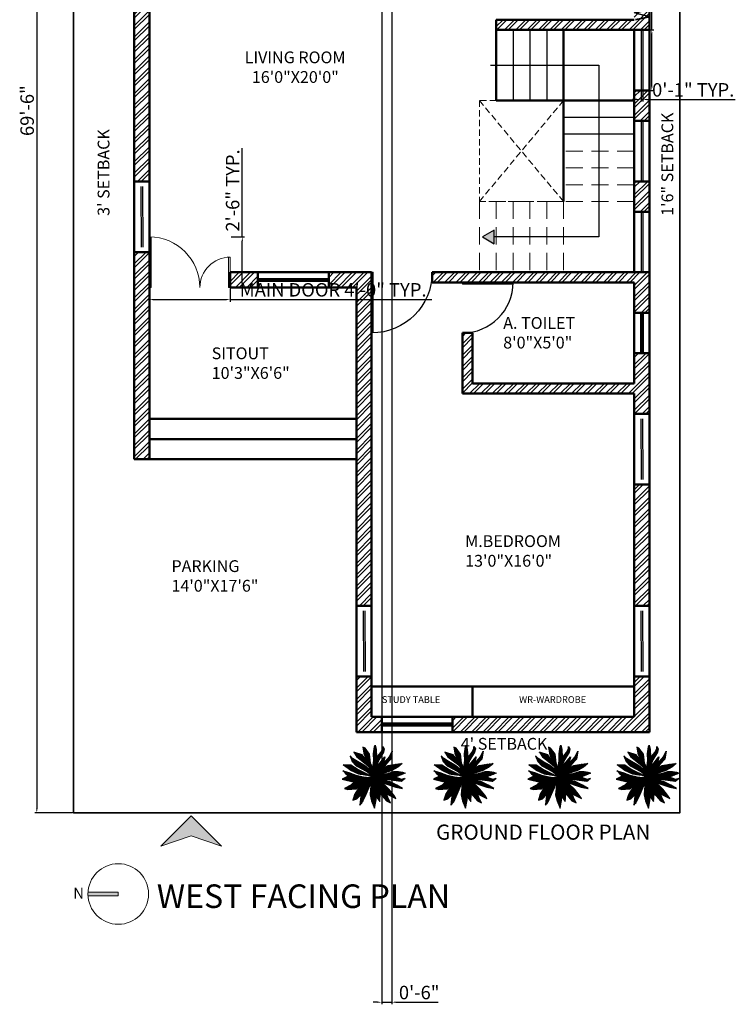
# Model space of a CAD drawing. Units: inches. Extents: x 1986 to 21484, y -1816 to 2016.
# Tile 46 of 85: x 3507 to 3932, y 953 to 1538. Entities that reach past the tile are written whole.
import ezdxf

# ---------------------------------------------------------------- set-up
doc = ezdxf.new("R2010")
doc.units = ezdxf.units.IN
doc.linetypes.add('DASHED', pattern=[19.05, 12.7, -6.35])
for name, color, linetype, lineweight in [('A-ANNO-DIMS', 2, 'Continuous', 18), ('A-ANNO-SYMB', 1, 'Continuous', 18), ('A-ANNO-TEXT', 7, 'Continuous', 18), ('A-AREA-IDEN', 3, 'Continuous', 18), ('A-DOOR', 3, 'Continuous', 25), ('A-FLOR-STRS', 7, 'Continuous', 25), ('A-FLOR-STRS-OVHD', 8, 'DASHED', 18), ('A-FURN', 8, 'Continuous', 18), ('A-GLAZ', 4, 'Continuous', 25), ('A-WALL', 7, 'Continuous', 50), ('A-WALL-PATT', 8, 'Continuous', 13), ('C-PROP', 7, 'Continuous', 35), ('L-PLNT', 84, 'Continuous', 13), ('vfolhas', 114, 'Continuous', 5)]:
    doc.layers.add(name, color=color, linetype=linetype, lineweight=lineweight)
for name, color, linetype in [('vfolha', 72, 'Continuous'), ('vfolha2', 110, 'Continuous'), ('vfolhas2', 102, 'Continuous')]:
    doc.layers.add(name, color=color, linetype=linetype)
doc.styles.get("Standard").update_dxf_attribs({"font": 'arial.ttf'})
doc.dimstyles.new('ISO-25', dxfattribs={"dimtxt": 8, "dimasz": 2.5, "dimexe": 1.25, "dimexo": 0.625, "dimtad": 1, "dimdec": 1, "dimlunit": 3, "dimtxsty": 'Standard', "dimcen": 2.5, "dimadec": 0, "dimazin": 0, "dimtfac": 1, "dimtdec": 1, "dimtmove": 0, "dimatfit": 3, "dimfxl": 1, "dimarcsym": 0})
pattern_1 = [(45, (-2446.5133113, 50.986076), (-0.004419417382, 0.004419417382), [])]

# ---------------------------------------------------------------- blocks, each defined once
blk = doc.blocks.new('*D32')
at = {"layer": 'A-ANNO-DIMS', "color": 0, "lineweight": -2, "transparency": 16777216}
for p, q in [((3538.28, 1900.75), (3515.81, 1900.75)), ((3517.06, 1898.25), (3517.06, 1069.25)), ((3538.28, 1066.75), (3515.81, 1066.75))]:
    blk.add_line(p, q, dxfattribs=at)
at = {"layer": 'A-ANNO-DIMS', "color": 0, "transparency": 16777216}
for points in [[(3516.64, 1898.25), (3517.47, 1898.25), (3517.06, 1900.75)], [(3516.64, 1069.25), (3517.47, 1069.25), (3517.06, 1066.75)]]:
    blk.add_solid(points, dxfattribs=at)
at = {"layer": 'Defpoints', "color": 0, "transparency": 16777216}
for p in [(3538.91, 1900.75), (3517.06, 1066.75), (3538.91, 1066.75)]:
    blk.add_point(p, dxfattribs=at)
at = {"layer": 'A-ANNO-DIMS', "color": 0, "transparency": 16777216, "insert": (3512.35, 1483.75), "char_height": 8, "attachment_point": 5, "rotation": 90}
blk.add_mtext('69\'-6"', dxfattribs=at)
blk = doc.blocks.new('arbusto_PB_verde_grande')
at = {"layer": 'vfolha2'}
h = blk.add_hatch(dxfattribs=at)
h.set_pattern_fill('ANSI31', color=256, scale=0.05, style=0)
h.set_pattern_definition(pattern_1)
h.paths.add_polyline_path([(0.029, 0.357), (0, 0.09), (0.026, -0.039), (0.047, 0.062), (0.062, 0.097), (0.094, 0.266), (0.1, 0.435), (0.088, 0.613), (0.064, 0.723), (0.05, 0.685), (0.024, 0.513)])
h.paths.add_polyline_path([(0.301, 0.438), (0.142, 0.249), (0.267, 0.3)])
h.paths.add_polyline_path([(0.38, 0.228), (0.237, 0.152), (0.184, 0.094), (0.111, 0.044), (0.026, -0.039), (0.281, 0.047), (0.368, 0.078), (0.468, 0.112), (0.611, 0.194), (0.716, 0.278), (0.558, 0.259)])
h.paths.add_polyline_path([(0.561, -0.294), (0.728, -0.326), (0.59, -0.241), (0.43, -0.16), (0.026, -0.039), (0.149, -0.141), (0.188, -0.166), (0.415, -0.244)])
h.paths.add_polyline_path([(-0.274, -0.448), (-0.304, -0.726), (-0.239, -0.642), (-0.155, -0.457), (0.026, -0.039), (-0.163, -0.254)])
h.paths.add_polyline_path([(-0.52, -0.247), (-0.677, -0.326), (-0.596, -0.351), (-0.406, -0.329), (-0.21, -0.21), (0.026, -0.039), (-0.149, -0.066), (-0.315, -0.091), (-0.415, -0.15)])
h.paths.add_polyline_path([(-0.525, 0.25), (-0.709, 0.247), (-0.52, 0.109), (-0.33, 0.022), (-0.076, -0.013), (-0.042, -0.021), (-0.35, 0.131)])
h = blk.add_hatch(dxfattribs=at)
h.set_pattern_fill('ANSI31', color=256, scale=0.05, style=0)
h.set_pattern_definition(pattern_1)
h.paths.add_polyline_path([(-0.19, 0.297), (-0.086, 0.202), (-0.108, 0.25), (-0.132, 0.319), (-0.251, 0.485), (-0.45, 0.551), (-0.379, 0.438)])
h.paths.add_polyline_path([(0.079, -0.407), (0.082, -0.506), (0.173, -0.635), (0.184, -0.442), (0.149, -0.292), (0.026, -0.039), (0.035, -0.254)])
at = {"layer": 'vfolhas'}
h = blk.add_hatch(dxfattribs=at)
h.set_pattern_fill('ANSI31', color=256, scale=0.05, style=0)
h.set_pattern_definition(pattern_1)
h.paths.add_polyline_path([(-0.073, 0.507), (-0.181, 0.651), (-0.233, 0.673), (-0.207, 0.532), (-0.108, 0.25), (0.026, -0.039), (0, 0.09), (0.008, 0.162), (-0.049, 0.291)])
h.paths.add_polyline_path([(0.099, 0.419), (0.094, 0.266), (0.079, 0.188), (0.155, 0.369), (0.266, 0.551), (0.284, 0.635), (0.249, 0.688), (0.251, 0.635), (0.202, 0.544)])
h.paths.add_polyline_path([(0.123, 0.241), (0.047, 0.062), (0.026, -0.039), (0.111, 0.044), (0.184, 0.094), (0.275, 0.194), (0.322, 0.253), (0.441, 0.385), (0.476, 0.579), (0.418, 0.453), (0.289, 0.31)])
h.paths.add_polyline_path([(0.581, -0.038), (0.707, 0.015), (0.786, 0.047), (0.748, 0.065), (0.628, 0.084), (0.526, 0.09), (0.397, 0.044), (0.026, -0.039), (0.257, -0.032), (0.438, -0.035)])
h.paths.add_polyline_path([(0.52, -0.036), (0.438, -0.035), (0.257, -0.032), (0.026, -0.039), (0.18, -0.085), (0.538, -0.132), (0.695, -0.154), (0.786, -0.079), (0.704, -0.1)])
h.paths.add_polyline_path([(0.272, -0.219), (0.149, -0.141), (0.026, -0.039), (0.158, -0.31), (0.295, -0.426), (0.418, -0.492), (0.564, -0.567), (0.511, -0.485), (0.395, -0.341)])
h.paths.add_polyline_path([(-0.058, -0.476), (-0.023, -0.62), (0.047, -0.801), (0.085, -0.598), (0.079, -0.407), (0.035, -0.254), (0.026, -0.039), (-0.038, -0.26)])
h.paths.add_polyline_path([(-0.242, 0.141), (-0.111, 0.069), (0.026, -0.039), (-0.042, 0.109), (-0.21, 0.238), (-0.365, 0.331), (-0.479, 0.403), (-0.543, 0.463), (-0.49, 0.331), (-0.394, 0.222)])
h = blk.add_hatch(dxfattribs=at)
h.set_pattern_fill('ANSI31', color=256, scale=0.05, style=0)
h.set_pattern_definition(pattern_1)
h.paths.add_polyline_path([(-0.572, 0.062), (-0.715, 0.103), (-0.677, 0.081), (-0.628, 0.015), (-0.563, -0.041), (-0.265, -0.083), (-0.149, -0.066), (-0.102, -0.059), (-0.204, -0.047), (-0.403, -0.003)])
h.paths.add_polyline_path([(-0.563, -0.041), (-0.583, -0.024), (-0.73, -0.097), (-0.433, -0.168), (-0.415, -0.15), (-0.315, -0.091), (-0.265, -0.083)])
h.paths.add_polyline_path([(-0.277, -0.473), (-0.274, -0.448), (-0.163, -0.254), (0.026, -0.039), (-0.21, -0.21), (-0.267, -0.245), (-0.365, -0.357), (-0.429, -0.463), (-0.476, -0.604), (-0.379, -0.576)])
h = blk.add_hatch(dxfattribs=at)
h.set_pattern_fill('ANSI31', color=256, scale=0.05, style=0)
h.set_pattern_definition(pattern_1)
h.paths.add_polyline_path([(0.336, -0.623), (0.433, -0.673), (0.395, -0.595), (0.33, -0.445), (0.295, -0.426), (0.158, -0.31), (0.149, -0.292), (0.184, -0.442)])
at = {"layer": 'vfolha'}
for p, q in [((0.026, -0.039), (-0.149, -0.066)), ((0.026, -0.039), (-0.038, -0.26)), ((0.035, -0.254), (0.026, -0.039)), ((0.538, -0.132), (0.18, -0.085)), ((0.395, -0.341), (0.272, -0.219)), ((0.52, -0.036), (0.704, -0.1)), ((0.695, -0.154), (0.538, -0.132)), ((0.786, -0.079), (0.695, -0.154)), ((0.704, -0.1), (0.786, -0.079)), ((-0.267, -0.245), (-0.365, -0.357)), ((-0.038, -0.26), (-0.058, -0.476)), ((0.079, -0.407), (0.035, -0.254)), ((0.085, -0.598), (0.079, -0.407)), ((0.158, -0.31), (0.295, -0.426)), ((0.295, -0.426), (0.418, -0.492)), ((0.511, -0.485), (0.395, -0.341)), ((-0.023, -0.62), (0.047, -0.801)), ((0.047, -0.801), (0.085, -0.598)), ((0.418, -0.492), (0.564, -0.567)), ((0.564, -0.567), (0.511, -0.485))]:
    blk.add_line(p, q, dxfattribs=at)
at = {"layer": 'vfolha2'}
for p, q in [((0.05, 0.685), (0.064, 0.723)), ((0.064, 0.723), (0.088, 0.613)), ((-0.45, 0.551), (-0.379, 0.438)), ((-0.251, 0.485), (-0.45, 0.551)), ((-0.132, 0.319), (-0.251, 0.485)), ((0.024, 0.513), (0.05, 0.685)), ((0.029, 0.357), (0.024, 0.513)), ((0.088, 0.613), (0.1, 0.435)), ((-0.709, 0.247), (-0.525, 0.25)), ((-0.52, 0.109), (-0.709, 0.247)), ((-0.525, 0.25), (-0.35, 0.131)), ((-0.379, 0.438), (-0.19, 0.297)), ((-0.19, 0.297), (-0.082, 0.199)), ((0, 0.09), (0.029, 0.357)), ((0.1, 0.435), (0.094, 0.266)), ((0.143, 0.25), (0.301, 0.438)), ((0.301, 0.438), (0.266, 0.297)), ((0.38, 0.228), (0.558, 0.259)), ((0.558, 0.259), (0.716, 0.278)), ((0.716, 0.278), (0.611, 0.194)), ((-0.33, 0.022), (-0.52, 0.109)), ((-0.35, 0.131), (-0.042, -0.021)), ((-0.076, -0.013), (-0.33, 0.022)), ((0.026, -0.039), (0, 0.09)), ((0.281, 0.047), (0.026, -0.039)), ((0.237, 0.152), (0.38, 0.228)), ((0.368, 0.078), (0.281, 0.047)), ((0.611, 0.194), (0.468, 0.112)), ((-0.415, -0.15), (-0.52, -0.247)), ((-0.315, -0.091), (-0.415, -0.15)), ((-0.406, -0.329), (-0.21, -0.21)), ((-0.149, -0.066), (-0.315, -0.091)), ((-0.21, -0.21), (0.026, -0.039)), ((0.026, -0.039), (-0.163, -0.254)), ((-0.155, -0.457), (0.026, -0.039)), ((0.43, -0.16), (0.026, -0.039)), ((0.026, -0.039), (0.158, -0.31)), ((0.188, -0.166), (0.415, -0.244)), ((0.59, -0.241), (0.43, -0.16)), ((-0.52, -0.247), (-0.677, -0.326)), ((-0.677, -0.326), (-0.596, -0.351)), ((-0.596, -0.351), (-0.406, -0.329)), ((-0.274, -0.448), (-0.304, -0.726)), ((-0.163, -0.254), (-0.274, -0.448)), ((0.184, -0.442), (0.149, -0.292)), ((0.173, -0.635), (0.184, -0.442)), ((0.415, -0.244), (0.561, -0.294)), ((0.561, -0.294), (0.728, -0.326)), ((0.728, -0.326), (0.59, -0.241)), ((-0.304, -0.726), (-0.239, -0.642)), ((0.082, -0.506), (0.173, -0.635))]:
    blk.add_line(p, q, dxfattribs=at)
at = {"layer": 'vfolhas2'}
for p, q in [((-0.233, 0.673), (-0.207, 0.532)), ((-0.181, 0.651), (-0.233, 0.673)), ((-0.207, 0.532), (-0.108, 0.25)), ((-0.073, 0.507), (-0.181, 0.651)), ((-0.049, 0.291), (-0.073, 0.507)), ((0.099, 0.419), (0.202, 0.544)), ((0.266, 0.551), (0.155, 0.369)), ((0.202, 0.544), (0.251, 0.635)), ((0.251, 0.635), (0.249, 0.688)), ((0.249, 0.688), (0.284, 0.635)), ((0.284, 0.635), (0.266, 0.551)), ((0.418, 0.453), (0.476, 0.579)), ((0.476, 0.579), (0.441, 0.385)), ((-0.543, 0.463), (-0.49, 0.331)), ((-0.479, 0.403), (-0.543, 0.463)), ((-0.49, 0.331), (-0.394, 0.222)), ((-0.365, 0.331), (-0.479, 0.403)), ((-0.21, 0.238), (-0.365, 0.331)), ((-0.108, 0.25), (0.026, -0.039)), ((0.008, 0.162), (-0.049, 0.291)), ((0.047, 0.062), (0.123, 0.241)), ((0.094, 0.266), (0.062, 0.097)), ((0.155, 0.369), (0.078, 0.186)), ((0.123, 0.241), (0.289, 0.31)), ((0.322, 0.253), (0.275, 0.194)), ((0.289, 0.31), (0.418, 0.453)), ((0.441, 0.385), (0.322, 0.253)), ((-0.677, 0.081), (-0.715, 0.103)), ((-0.715, 0.103), (-0.572, 0.062)), ((-0.628, 0.015), (-0.677, 0.081)), ((-0.563, -0.041), (-0.628, 0.015)), ((-0.572, 0.062), (-0.403, -0.003)), ((-0.394, 0.222), (-0.242, 0.141)), ((-0.242, 0.141), (-0.111, 0.069)), ((-0.042, 0.109), (-0.21, 0.238)), ((-0.111, 0.069), (0.026, -0.039)), ((0.026, -0.039), (0.047, 0.062)), ((0.026, -0.039), (0.397, 0.044)), ((0.111, 0.044), (0.026, -0.039)), ((0.184, 0.094), (0.111, 0.044)), ((0.275, 0.194), (0.184, 0.094)), ((0.468, 0.112), (0.368, 0.078)), ((0.397, 0.044), (0.526, 0.09)), ((0.526, 0.09), (0.628, 0.084)), ((0.707, 0.015), (0.581, -0.038)), ((0.628, 0.084), (0.748, 0.065)), ((0.786, 0.047), (0.707, 0.015)), ((0.748, 0.065), (0.786, 0.047)), ((-0.583, -0.024), (-0.73, -0.097)), ((-0.73, -0.097), (-0.433, -0.168)), ((-0.265, -0.083), (-0.563, -0.041)), ((-0.403, -0.003), (-0.204, -0.047)), ((-0.204, -0.047), (-0.098, -0.059)), ((0.026, -0.039), (-0.076, -0.013)), ((0.257, -0.032), (0.026, -0.039)), ((0.149, -0.141), (0.026, -0.039)), ((0.272, -0.219), (0.149, -0.141)), ((0.438, -0.035), (0.257, -0.032)), ((0.581, -0.038), (0.438, -0.035)), ((-0.429, -0.463), (-0.476, -0.604)), ((-0.365, -0.357), (-0.429, -0.463)), ((-0.379, -0.576), (-0.277, -0.473)), ((-0.239, -0.642), (-0.155, -0.457)), ((0.184, -0.442), (0.336, -0.623)), ((0.395, -0.595), (0.329, -0.442)), ((-0.476, -0.604), (-0.379, -0.576)), ((-0.058, -0.476), (-0.023, -0.62)), ((0.336, -0.623), (0.433, -0.673)), ((0.433, -0.673), (0.395, -0.595))]:
    blk.add_line(p, q, dxfattribs=at)
blk = doc.blocks.new('MD')
for p, q in [((1902.58, 1512.86), (1902.58, 1482.86)), ((1903.58, 1512.86), (1903.58, 1482.86)), ((1949.58, 1482.86), (1949.58, 1500.86)), ((1950.58, 1482.86), (1950.58, 1500.86)), ((1902.58, 1482.86), (1903.58, 1482.86)), ((1949.58, 1482.86), (1950.58, 1482.86))]:
    blk.add_line(p, q)
for centre, radius, start, end in [((1902.58, 1482.86), 30, 0, 90), ((1950.58, 1482.86), 18, 90, 180)]:
    blk.add_arc(centre, radius, start, end)
blk = doc.blocks.new('D2')
for p, q in [((1722.5, 1505.46), (1722.5, 1475.46)), ((1723.5, 1505.46), (1723.5, 1475.46)), ((1722.5, 1475.46), (1723.5, 1475.46))]:
    blk.add_line(p, q)
blk.add_arc((1722.5, 1475.46), 30, 0, 90)
blk = doc.blocks.new('D1')
for p, q in [((1805.96, 1500.36), (1805.96, 1464.36)), ((1806.96, 1500.36), (1806.96, 1464.36)), ((1805.96, 1464.36), (1806.96, 1464.36))]:
    blk.add_line(p, q)
blk.add_arc((1805.96, 1464.36), 36, 0, 90)
blk = doc.blocks.new('WIN-36')
for p, q in [((0, 36), (0, 0)), ((0, 36), (0, 0)), ((1, 36), (1, 0))]:
    blk.add_line(p, q)
blk = doc.blocks.new('*D87')
at = {"layer": 'A-ANNO-DIMS', "color": 0, "lineweight": -2, "transparency": 16777216}
for p, q in [((3882.31, 1531.75), (3882.31, 1636.74)), ((3877.53, 1531.75), (3883.56, 1531.75)), ((3882.31, 1498.25), (3882.31, 1529.25)), ((3877.53, 1495.75), (3883.56, 1495.75))]:
    blk.add_line(p, q, dxfattribs=at)
at = {"layer": 'A-ANNO-DIMS', "color": 0, "transparency": 16777216}
for points in [[(3881.89, 1529.25), (3882.72, 1529.25), (3882.31, 1531.75)], [(3881.89, 1498.25), (3882.72, 1498.25), (3882.31, 1495.75)]]:
    blk.add_solid(points, dxfattribs=at)
at = {"layer": 'Defpoints', "color": 0, "transparency": 16777216}
for p in [(3876.91, 1531.75), (3882.31, 1531.75), (3876.91, 1495.75)]:
    blk.add_point(p, dxfattribs=at)
at = {"layer": 'A-ANNO-DIMS', "color": 0, "transparency": 16777216, "insert": (3877.54, 1585.49), "char_height": 8, "attachment_point": 5, "rotation": 90}
blk.add_mtext('WINDOW 3\'-0" TYP.', dxfattribs=at)
blk = doc.blocks.new('*D88')
at = {"layer": 'A-ANNO-DIMS', "color": 0, "lineweight": -2, "transparency": 16777216}
for p, q in [((3875.91, 1495.13), (3875.91, 1489.1)), ((3876.91, 1495.13), (3876.91, 1489.1)), ((3873.41, 1490.35), (3870.91, 1490.35)), ((3875.91, 1490.35), (3876.91, 1490.35)), ((3879.41, 1490.35), (3931.92, 1490.35))]:
    blk.add_line(p, q, dxfattribs=at)
at = {"layer": 'A-ANNO-DIMS', "color": 0, "transparency": 16777216}
for points in [[(3873.41, 1490.77), (3873.41, 1489.94), (3875.91, 1490.35)], [(3879.41, 1490.77), (3879.41, 1489.94), (3876.91, 1490.35)]]:
    blk.add_solid(points, dxfattribs=at)
at = {"layer": 'Defpoints', "color": 0, "transparency": 16777216}
for p in [(3875.91, 1495.75), (3876.91, 1495.75), (3876.91, 1490.35)]:
    blk.add_point(p, dxfattribs=at)
at = {"layer": 'A-ANNO-DIMS', "color": 0, "transparency": 16777216, "insert": (3906.91, 1495.06), "char_height": 8, "attachment_point": 5}
blk.add_mtext('0\'-1" TYP.', dxfattribs=at)
blk = doc.blocks.new('*D93')
at = {"layer": 'A-ANNO-DIMS', "color": 0, "lineweight": -2, "transparency": 16777216}
for p, q in [((3583.91, 1378.13), (3583.91, 1370.3)), ((3631.91, 1378.13), (3631.91, 1370.3)), ((3586.41, 1371.55), (3629.41, 1371.55)), ((3631.91, 1371.55), (3751.73, 1371.55))]:
    blk.add_line(p, q, dxfattribs=at)
at = {"layer": 'A-ANNO-DIMS', "color": 0, "transparency": 16777216}
for points in [[(3586.41, 1371.97), (3586.41, 1371.14), (3583.91, 1371.55)], [(3629.41, 1371.97), (3629.41, 1371.14), (3631.91, 1371.55)]]:
    blk.add_solid(points, dxfattribs=at)
at = {"layer": 'Defpoints', "color": 0, "transparency": 16777216}
for p in [(3583.91, 1378.75), (3631.91, 1378.75), (3631.91, 1371.55)]:
    blk.add_point(p, dxfattribs=at)
at = {"layer": 'A-ANNO-DIMS', "color": 0, "transparency": 16777216, "insert": (3693.07, 1376.32), "char_height": 8, "attachment_point": 5}
blk.add_mtext('MAIN DOOR 4\'-0" TYP.', dxfattribs=at)
blk = doc.blocks.new('*D94')
at = {"layer": 'A-ANNO-DIMS', "color": 0, "lineweight": -2, "transparency": 16777216}
for p, q in [((3639.11, 1408.75), (3639.11, 1461.4)), ((3632.53, 1408.75), (3640.36, 1408.75)), ((3639.11, 1381.25), (3639.11, 1406.25)), ((3632.53, 1378.75), (3640.36, 1378.75))]:
    blk.add_line(p, q, dxfattribs=at)
at = {"layer": 'A-ANNO-DIMS', "color": 0, "transparency": 16777216}
for points in [[(3638.69, 1406.25), (3639.52, 1406.25), (3639.11, 1408.75)], [(3638.69, 1381.25), (3639.52, 1381.25), (3639.11, 1378.75)]]:
    blk.add_solid(points, dxfattribs=at)
at = {"layer": 'Defpoints', "color": 0, "transparency": 16777216}
for p in [(3631.91, 1408.75), (3639.11, 1408.75), (3631.91, 1378.75)]:
    blk.add_point(p, dxfattribs=at)
at = {"layer": 'A-ANNO-DIMS', "color": 0, "transparency": 16777216, "insert": (3634.4, 1436.33), "char_height": 8, "attachment_point": 5, "rotation": 90}
blk.add_mtext('2\'-6" TYP.', dxfattribs=at)
blk = doc.blocks.new('*D128')
at = {"layer": 'A-ANNO-DIMS', "color": 0, "lineweight": -2, "transparency": 16777216}
for p, q in [((3721.91, 1627.13), (3721.91, 953.11)), ((3727.91, 1627.13), (3727.91, 953.11)), ((3719.41, 954.36), (3716.91, 954.36)), ((3721.91, 954.36), (3727.91, 954.36)), ((3730.41, 954.36), (3755.42, 954.36))]:
    blk.add_line(p, q, dxfattribs=at)
at = {"layer": 'A-ANNO-DIMS', "color": 0, "transparency": 16777216}
for points in [[(3719.41, 954.78), (3719.41, 953.95), (3721.91, 954.36)], [(3730.41, 954.78), (3730.41, 953.95), (3727.91, 954.36)]]:
    blk.add_solid(points, dxfattribs=at)
at = {"layer": 'Defpoints', "color": 0, "transparency": 16777216}
for p in [(3721.91, 1627.75), (3727.91, 1627.75), (3727.91, 954.36)]:
    blk.add_point(p, dxfattribs=at)
at = {"layer": 'A-ANNO-DIMS', "color": 0, "transparency": 16777216, "insert": (3744.17, 959.07), "char_height": 8, "attachment_point": 5}
blk.add_mtext('0\'-6"', dxfattribs=at)

msp = doc.modelspace()

# ---------------------------------------------------------------- hatches: boundary and pattern name
at = {"layer": 'A-ANNO-SYMB'}
h = msp.add_hatch(color=256, dxfattribs=at)
h.dxf.hatch_style = 1
h.paths.add_polyline_path([(3608.7, 1065.1), (3590.7, 1047.1), (3608.7, 1053.1), (3626.7, 1047.1)])
h = msp.add_hatch(color=256, dxfattribs=at)
h.dxf.hatch_style = 1
h.paths.add_polyline_path([(3547.49, 1019.61, 0.013897), (3547.46, 1018.61, 0.013897), (3547.49, 1017.61), (3565.46, 1017.61), (3565.46, 1019.61)])
at = {"layer": 'A-FLOR-STRS'}
h = msp.add_hatch(color=256, dxfattribs=at)
h.dxf.hatch_style = 1
h.paths.add_polyline_path([(3781.75, 1408.75), (3788.7, 1404.74), (3788.7, 1412.77)])
at = {"layer": 'A-WALL-PATT'}
h = msp.add_hatch(dxfattribs=at)
h.set_pattern_fill('ANSI32', color=256, scale=0.5)
h.paths.add_polyline_path([(3631.91, 1852.75), (3574.91, 1852.75), (3574.91, 1753.75), (3583.91, 1753.75), (3583.91, 1843.75), (3631.91, 1843.75)])
h.paths.add_polyline_path([(3727.91, 1852.75), (3673.91, 1852.75), (3673.91, 1843.75), (3721.91, 1843.75), (3721.91, 1627.75), (3727.91, 1627.75)])
h.paths.add_polyline_path([(3880.91, 1852.75), (3757.91, 1852.75), (3757.91, 1843.75), (3871.91, 1843.75), (3871.91, 1795.75), (3775.91, 1795.75), (3775.91, 1813.75), (3769.91, 1813.75), (3769.91, 1789.75), (3871.91, 1789.75), (3871.91, 1741.75), (3880.91, 1741.75)])
h.paths.add_polyline_path([(3880.91, 1705.75), (3871.91, 1705.75), (3871.91, 1600.75), (3880.91, 1600.75)])
h.paths.add_polyline_path([(3685.91, 1687.75), (3583.91, 1687.75), (3583.91, 1711.75), (3574.91, 1711.75), (3574.91, 1669.75), (3583.91, 1669.75), (3583.91, 1681.75), (3673.91, 1681.75), (3673.91, 1663.75), (3679.91, 1663.75), (3679.91, 1681.75), (3685.91, 1681.75)])
h.paths.add_polyline_path([(3583.91, 1399.75), (3574.91, 1399.75), (3574.91, 1276.75), (3583.91, 1276.75)])
h.paths.add_polyline_path([(3648.41, 1387.75), (3631.91, 1387.75), (3631.91, 1378.75), (3648.41, 1378.75)])
h.paths.add_polyline_path([(3715.91, 1387.75), (3690.41, 1387.75), (3690.41, 1378.75), (3706.91, 1378.75), (3706.91, 1189.75), (3715.91, 1189.75)])
h.paths.add_polyline_path([(3880.91, 1387.75), (3871.91, 1387.75), (3751.91, 1387.75), (3751.91, 1381.75), (3871.91, 1381.75), (3871.91, 1363.75), (3880.91, 1363.75)])
h.paths.add_polyline_path([(3880.91, 1441.75), (3871.91, 1441.75), (3871.91, 1423.75), (3880.91, 1423.75)])
h.paths.add_polyline_path([(3880.91, 1495.75), (3871.91, 1495.75), (3871.91, 1477.75), (3880.91, 1477.75)])
h.paths.add_polyline_path([(3880.91, 1339.75), (3871.91, 1339.75), (3871.91, 1321.75), (3775.91, 1321.75), (3775.91, 1351.75), (3769.91, 1351.75), (3769.91, 1315.75), (3871.91, 1315.75), (3871.91, 1303.75), (3880.91, 1303.75)])
h.paths.add_polyline_path([(3880.91, 1261.75), (3871.91, 1261.75), (3871.91, 1189.75), (3880.91, 1189.75)])
h.paths.add_polyline_path([(3880.91, 1147.75), (3871.91, 1147.75), (3871.91, 1123.75), (3763.91, 1123.75), (3763.91, 1114.75), (3880.91, 1114.75)])
h.paths.add_polyline_path([(3721.91, 1123.75), (3715.91, 1123.75), (3715.91, 1147.75), (3706.91, 1147.75), (3706.91, 1114.75), (3721.91, 1114.75)])
h.paths.add_polyline_path([(3880.91, 1564.75), (3871.91, 1564.75), (3871.91, 1537.75), (3789.91, 1537.75), (3789.91, 1531.75), (3871.91, 1531.75), (3880.91, 1531.75)])
h.paths.add_polyline_path([(3583.91, 1627.75), (3679.91, 1627.75), (3679.91, 1633.75), (3649.91, 1633.75), (3583.91, 1633.75), (3583.91, 1645.75), (3574.91, 1645.75), (3574.91, 1441.75), (3583.91, 1441.75)])
h.paths.add_polyline_path([(3733.26, 1736.83), (3733.26, 1685.78), (3741.8, 1685.78), (3741.8, 1736.83)], flags=9)
h.paths.add_polyline_path([(3763.81, 1864.73), (3812.77, 1864.73), (3812.77, 1891.35), (3763.81, 1891.35)], flags=9)
h.paths.add_polyline_path([(3797.97, 1806.84), (3841.79, 1806.84), (3841.79, 1833.45), (3797.97, 1833.45)], flags=25)
h.paths.add_polyline_path([(3779.25, 1690.08), (3833.38, 1690.08), (3833.38, 1716.69), (3779.25, 1716.69)], flags=9)
h.paths.add_polyline_path([(3805.23, 1565.41), (3849.03, 1565.41), (3849.03, 1592.03), (3805.23, 1592.03)], flags=9)
h.paths.add_polyline_path([(3638.57, 1496.24), (3711.25, 1496.24), (3711.25, 1522.85), (3638.57, 1522.85)], flags=9)
h.paths.add_polyline_path([(3617.97, 1320.51), (3666.93, 1320.51), (3666.93, 1347.12), (3617.97, 1347.12)], flags=9)
h.paths.add_polyline_path([(3768.51, 1208.98), (3836.51, 1208.98), (3836.51, 1235.59), (3768.51, 1235.59)], flags=9)
h.paths.add_polyline_path([(3791.7, 1338.54), (3844.53, 1338.54), (3844.53, 1365.15), (3791.7, 1365.15)], flags=9)
h.paths.add_polyline_path([(3614.85, 1758.76), (3671.08, 1758.76), (3671.08, 1785.38), (3614.85, 1785.38)], flags=9)
h.paths.add_polyline_path([(3603.38, 1642.68), (3655.11, 1642.68), (3655.11, 1669.29), (3603.38, 1669.29)], flags=9)

# ---------------------------------------------------------------- linework, layer by layer
at = {"layer": 'A-ANNO-SYMB'}
for p, q in [((3608.7, 1065.1), (3590.7, 1047.1)), ((3608.7, 1065.1), (3626.7, 1047.1)), ((3590.7, 1047.1), (3608.7, 1053.1)), ((3608.7, 1053.1), (3590.7, 1047.1)), ((3626.7, 1047.1), (3608.7, 1053.1)), ((3608.7, 1053.1), (3626.7, 1047.1)), ((3565.46, 1019.61), (3547.46, 1019.61)), ((3565.46, 1017.61), (3547.46, 1017.61)), ((3565.46, 1019.61), (3565.46, 1017.61))]:
    msp.add_line(p, q, dxfattribs=at)
msp.add_circle((3565.46, 1018.61), 18, dxfattribs=at)
at = {"layer": 'A-FLOR-STRS'}
for p, q in [((3799.91, 1531.75), (3799.91, 1489.75)), ((3809.91, 1531.75), (3809.91, 1489.75)), ((3819.91, 1531.75), (3819.91, 1489.75)), ((3871.91, 1479.75), (3829.91, 1479.75)), ((3871.91, 1469.75), (3829.91, 1469.75))]:
    msp.add_line(p, q, dxfattribs=at)
msp.add_lwpolyline([(3786.49, 1510.75), (3850.91, 1510.75), (3850.91, 1408.75), (3788.7, 1408.75)], dxfattribs=at)
msp.add_lwpolyline([(3781.75, 1408.75), (3788.7, 1404.74), (3788.7, 1412.77)], close=True, dxfattribs=at)
at = {"layer": 'A-FLOR-STRS-OVHD', "ltscale": 0.3}
for p, q in [((3779.91, 1489.75), (3829.91, 1429.75)), ((3779.91, 1429.75), (3829.91, 1489.75))]:
    msp.add_line(p, q, dxfattribs=at)
at = {"layer": 'A-FLOR-STRS-OVHD', "ltscale": 0.8}
for p, q in [((3871.91, 1459.75), (3829.91, 1459.75)), ((3871.91, 1449.75), (3829.91, 1449.75)), ((3871.91, 1439.75), (3829.91, 1439.75)), ((3779.91, 1429.75), (3779.91, 1387.75)), ((3871.91, 1429.75), (3779.91, 1429.75)), ((3789.91, 1429.75), (3789.91, 1387.75)), ((3799.91, 1429.75), (3799.91, 1387.75)), ((3809.91, 1429.75), (3809.91, 1387.75)), ((3819.91, 1429.75), (3819.91, 1387.75)), ((3829.91, 1429.75), (3829.91, 1387.75))]:
    msp.add_line(p, q, dxfattribs=at)
at = {"layer": 'A-FLOR-STRS-OVHD', "ltscale": 0.3}
msp.add_lwpolyline([(3779.91, 1429.75), (3829.91, 1429.75), (3829.91, 1489.75), (3779.91, 1489.75)], close=True, dxfattribs=at)
at = {"layer": 'A-WALL'}
for p, q in [((3880.91, 1900.75), (3880.91, 1114.75)), ((3574.91, 1276.75), (3574.91, 1852.75)), ((3583.91, 1276.75), (3583.91, 1627.75)), ((3789.91, 1537.75), (3789.91, 1489.75)), ((3789.91, 1537.75), (3871.91, 1537.75)), ((3789.91, 1531.75), (3871.91, 1531.75)), ((3829.91, 1531.75), (3829.91, 1429.75)), ((3871.91, 1531.75), (3871.91, 1387.75)), ((3871.91, 1531.75), (3880.91, 1531.75)), ((3871.91, 1495.75), (3880.91, 1495.75)), ((3871.91, 1489.75), (3789.91, 1489.75)), ((3871.91, 1477.75), (3880.91, 1477.75)), ((3574.91, 1441.75), (3583.91, 1441.75)), ((3871.91, 1441.75), (3880.91, 1441.75)), ((3871.91, 1423.75), (3880.91, 1423.75)), ((3574.91, 1399.75), (3583.91, 1399.75)), ((3631.91, 1378.75), (3631.91, 1387.75)), ((3631.91, 1387.75), (3715.91, 1387.75)), ((3648.41, 1378.75), (3648.41, 1387.75)), ((3690.41, 1378.75), (3690.41, 1387.75)), ((3715.91, 1123.75), (3715.91, 1387.75)), ((3751.91, 1387.75), (3871.91, 1387.75)), ((3751.91, 1381.75), (3751.91, 1387.75)), ((3871.91, 1387.75), (3880.91, 1387.75)), ((3648.41, 1383.75), (3690.41, 1383.75)), ((3648.41, 1382.75), (3690.41, 1382.75)), ((3751.91, 1381.75), (3871.91, 1381.75)), ((3871.91, 1381.75), (3871.91, 1321.75)), ((3631.91, 1378.75), (3706.91, 1378.75)), ((3706.91, 1114.75), (3706.91, 1378.75)), ((3871.91, 1363.75), (3880.91, 1363.75)), ((3875.91, 1339.75), (3875.91, 1363.75)), ((3876.91, 1339.75), (3876.91, 1363.75)), ((3769.91, 1351.75), (3769.91, 1315.75)), ((3769.91, 1351.75), (3775.91, 1351.75)), ((3775.91, 1351.75), (3775.91, 1321.75)), ((3871.91, 1339.75), (3880.91, 1339.75)), ((3775.91, 1321.75), (3871.91, 1321.75)), ((3769.91, 1315.75), (3871.91, 1315.75)), ((3871.91, 1315.75), (3871.91, 1123.75)), ((3871.91, 1303.75), (3880.91, 1303.75)), ((3583.91, 1300.75), (3706.91, 1300.75)), ((3583.91, 1288.75), (3706.91, 1288.75)), ((3574.91, 1276.75), (3706.91, 1276.75)), ((3871.91, 1261.75), (3880.91, 1261.75)), ((3706.91, 1189.75), (3715.91, 1189.75)), ((3871.91, 1189.75), (3880.91, 1189.75)), ((3706.91, 1147.75), (3715.91, 1147.75)), ((3871.91, 1147.75), (3880.91, 1147.75)), ((3715.91, 1141.75), (3871.91, 1141.75)), ((3775.91, 1123.75), (3775.91, 1141.75)), ((3715.91, 1123.75), (3871.91, 1123.75)), ((3721.91, 1114.75), (3721.91, 1123.75)), ((3763.91, 1114.75), (3763.91, 1123.75)), ((3721.91, 1119.75), (3763.91, 1119.75)), ((3721.91, 1118.75), (3763.91, 1118.75)), ((3880.91, 1114.75), (3706.91, 1114.75))]:
    msp.add_line(p, q, dxfattribs=at)
at = {"layer": 'C-PROP'}
msp.add_lwpolyline([(3538.91, 1900.75), (3898.91, 1900.75), (3898.91, 1066.75), (3538.91, 1066.75)], close=True, dxfattribs=at)

# ---------------------------------------------------------------- block references
at = {"layer": 'A-DOOR', "xscale": -1, "rotation": 180}
msp.add_blockref('D1', (1909.94, 2852.11), dxfattribs=at)
at = {"layer": 'A-DOOR', "rotation": 270}
msp.add_blockref('D2', (2294.45, 3104.25), dxfattribs=at)
at = {"layer": 'A-FURN'}
msp.add_blockref('MD', (1681.32, -104.11), dxfattribs=at)
at = {"layer": 'A-GLAZ'}
for p in [(3875.91, 1495.75), (3875.91, 1441.75), (3875.91, 1387.75)]:
    msp.add_blockref('WIN-36', p, dxfattribs=at)
at = {"layer": 'A-GLAZ', "rotation": 0.302793432207276}
for p in [(3579, 1402.75), (3876, 1264.75), (3711, 1150.75), (3876, 1150.75)]:
    msp.add_blockref('WIN-36', p, dxfattribs=at)
at = {"layer": 'L-PLNT', "xscale": 24.60366729364114, "yscale": 24.60366729364114, "zscale": 24.60366729364114}
for p in [(3716.44, 1089.23), (3770.53, 1089.23), (3826.65, 1089.23), (3879.16, 1089.23)]:
    msp.add_blockref('arbusto_PB_verde_grande', p, dxfattribs=at)

# ---------------------------------------------------------------- texts
at = {"layer": 'A-ANNO-SYMB'}
msp.add_text('N ', height=6.465, dxfattribs=at).set_placement((3538.7, 1015.88))
at = {"layer": 'A-ANNO-TEXT', "char_height": 7, "attachment_point": 1, "rotation": 90}
for s, insert in [('{\\fTimes New Roman|b0|i0|c0|p18;1\'6" SETBACK}', (3888.05, 1421.26)), ("{\\fTimes New Roman|b0|i0|c0|p18;3' SETBACK}", (3553.21, 1421.26))]:
    msp.add_mtext_dynamic_manual_height_columns(s, width=105.6127, gutter_width=12.5, heights=[0], dxfattribs=dict(at, insert=insert))
at = {"layer": 'A-ANNO-TEXT', "attachment_point": 1}
for s, width, insert, char_height in [('{\\fTimes New Roman|b0|i0|c0|p18;STUDY TABLE}', 105.6127, (3722.01, 1136.07), 4), ('{\\fTimes New Roman|b0|i0|c0|p18;WR-WARDROBE}', 105.6127, (3803.52, 1136.07), 4), ("{\\fTimes New Roman|b0|i0|c0|p18;4' SETBACK}", 105.6127, (3768.85, 1111.29), 7), ('{\\fTimes New Roman|b0|i0|c0|p18;GROUND FLOOR PLAN}', 226.7688, (3754.19, 1059.84), 9), ('{\\fTimes New Roman|b0|i0|c0|p18;WEST FACING PLAN}', 226.7688, (3588.35, 1024.3), 14)]:
    msp.add_mtext_dynamic_manual_height_columns(s, width=width, gutter_width=12.5, heights=[0], dxfattribs=dict(at, insert=insert, char_height=char_height))
at = {"layer": 'A-AREA-IDEN', "char_height": 7, "attachment_point": 1}
for s, width, insert in [('{\\fTimes New Roman|b0|i0|c0|p18;LIVING ROOM\\P  16\'0"X20\'0"}', 122.2228, (3640.52, 1518.89)), ('{\\fTimes New Roman|b0|i0|c0|p18;A. TOILET\\P8\'0"X5\'0"}', 105.6127, (3794.07, 1361.19)), ('{\\fTimes New Roman|b0|i0|c0|p18;SITOUT\\P10\'3"X6\'6"}', 105.6127, (3620.93, 1343.16)), ('{\\fTimes New Roman|b0|i0|c0|p18;M.BEDROOM \\P13\'0"X16\'0"}', 105.6127, (3771.48, 1231.63)), ('{\\fTimes New Roman|b0|i0|c0|p18;PARKING\\P14\'0"X17\'6"}', 105.6127, (3597.05, 1216.8))]:
    msp.add_mtext_dynamic_manual_height_columns(s, width=width, gutter_width=12.5, heights=[0], dxfattribs=dict(at, insert=insert))

# ---------------------------------------------------------------- dimensions: what is measured, and where the dimension line sits
at = {"layer": 'A-ANNO-DIMS'}
dim = msp.add_linear_dim(base=(3517.06, 1066.75), p1=(3538.91, 1900.75), p2=(3538.91, 1066.75), angle=90, dimstyle='ISO-25', override={"dimclrd": 0, "dimclre": 0, "dimclrt": 0}, dxfattribs=at)
dim.commit()
dim.dimension.update_dxf_attribs({"geometry": '*D32', "text_midpoint": (3512.35, 1483.75)})
for base, p1, p2, text, picture, middle in [((3882.31, 1531.75), (3876.91, 1495.75), (3876.91, 1531.75), 'WINDOW <> TYP.', '*D87', (3877.54, 1585.49)), ((3639.11, 1408.75), (3631.91, 1378.75), (3631.91, 1408.75), '<> TYP.', '*D94', (3634.4, 1436.33))]:
    dim = msp.add_linear_dim(base=base, p1=p1, p2=p2, angle=90, text=text, dimstyle='ISO-25', override={"dimdec": 1, "dimrnd": 0, "dimzin": 1, "dimlunit": 4, "dimfrac": 2}, dxfattribs=at)
    dim.commit()
    dim.dimension.update_dxf_attribs({"geometry": picture, "text_midpoint": middle})
dim = msp.add_linear_dim(base=(3727.91, 954.36), p1=(3721.91, 1627.75), p2=(3727.91, 1627.75), dimstyle='ISO-25', override={"dimdec": 1, "dimlfac": 1, "dimrnd": 0, "dimzin": 1, "dimdsep": 46, "dimlunit": 4, "dimfrac": 2}, dxfattribs=at)
dim.commit()
dim.dimension.update_dxf_attribs({"geometry": '*D128', "text_midpoint": (3744.17, 959.07)})
for base, p1, p2, text, picture, middle in [((3876.91, 1490.35), (3875.91, 1495.75), (3876.91, 1495.75), '<> TYP.', '*D88', (3906.91, 1495.06)), ((3631.91, 1371.55), (3583.91, 1378.75), (3631.91, 1378.75), 'MAIN DOOR <> TYP.', '*D93', (3693.07, 1376.32))]:
    dim = msp.add_linear_dim(base=base, p1=p1, p2=p2, text=text, dimstyle='ISO-25', override={"dimdec": 1, "dimrnd": 0, "dimzin": 1, "dimlunit": 4, "dimfrac": 2}, dxfattribs=at)
    dim.commit()
    dim.dimension.update_dxf_attribs({"geometry": picture, "text_midpoint": middle})

doc.saveas('drawing.dxf')
